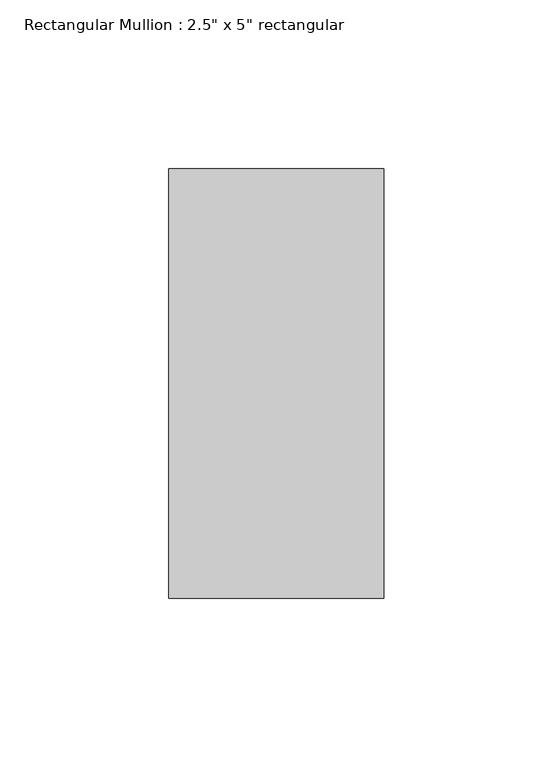
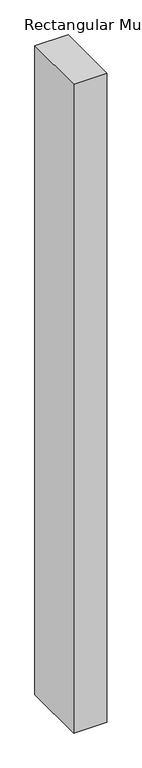
"""IFC4 building model written with IfcOpenShell, lengths in millimetres: member geometry."""

from ifc_helpers import new_model, si_unit, frame, origin, place, context, project, spatial, polyline, outline, extrude, source, transform, mapped, element, save


def member_44103a32(model_context):
    return source(origin(), model_context, "Body", "SweptSolid", [
        extrude(outline(polyline([(31.75, 63.5), (31.75, -63.5), (-31.75, -63.5), (-31.75, 63.5), (31.75, 63.5)])), frame((0.0, 0.0, -1301.75), z_axis=(0.0, 0.0, 1.0), x_axis=(1.0, 0.0, 0.0)), (0.0, 0.0, 1.0), 1301.75),
    ])


if __name__ == "__main__":
    model = new_model("IFC4")
    model_context = context("Model", 3, world=origin())
    ifc_project = project(units=[si_unit("LENGTHUNIT", "METRE", prefix="MILLI")], contexts=[model_context])
    site = spatial("IfcSite", under=ifc_project)
    building = spatial("IfcBuilding", under=site)
    placement = place(None, origin())
    member_shape = member_44103a32(model_context)
    element("IfcMember", 1, ObjectType="Rectangular Mullion : 2.5\" x 5\" rectangular", at=placement, inside=building, context=model_context, shape_type="MappedRepresentation", body=[
        mapped(member_shape, transform((0.0, 0.0, 0.0), x_axis=(1.0, 0.0, 0.0), y_axis=(0.0, 1.0, 0.0), z_axis=(0.0, 0.0, 1.0))),
    ])
    save(model, "model.ifc")

# Revit data of these elements
# Type "Rectangular Mullion : 2.5\" x 5\" rectangular"
#   built-in parameter 1007304 = 0.416667 (stored number, unit not read)
#   built-in parameter 1007301 = 0.104167 (stored number, unit not read)
#   built-in parameter 1007300 = 0.104167 (stored number, unit not read)
# Element 1 (IfcMember, "Rectangular Mullion : 2.5\" x 5\" rectangular")
#   Materials on its faces: "Aluminum"
# Materials
#   "Aluminum": class "Metal", colour RGB 247 247 247, transparency 0, Description = "Aluminum 6061", Cost = 0
